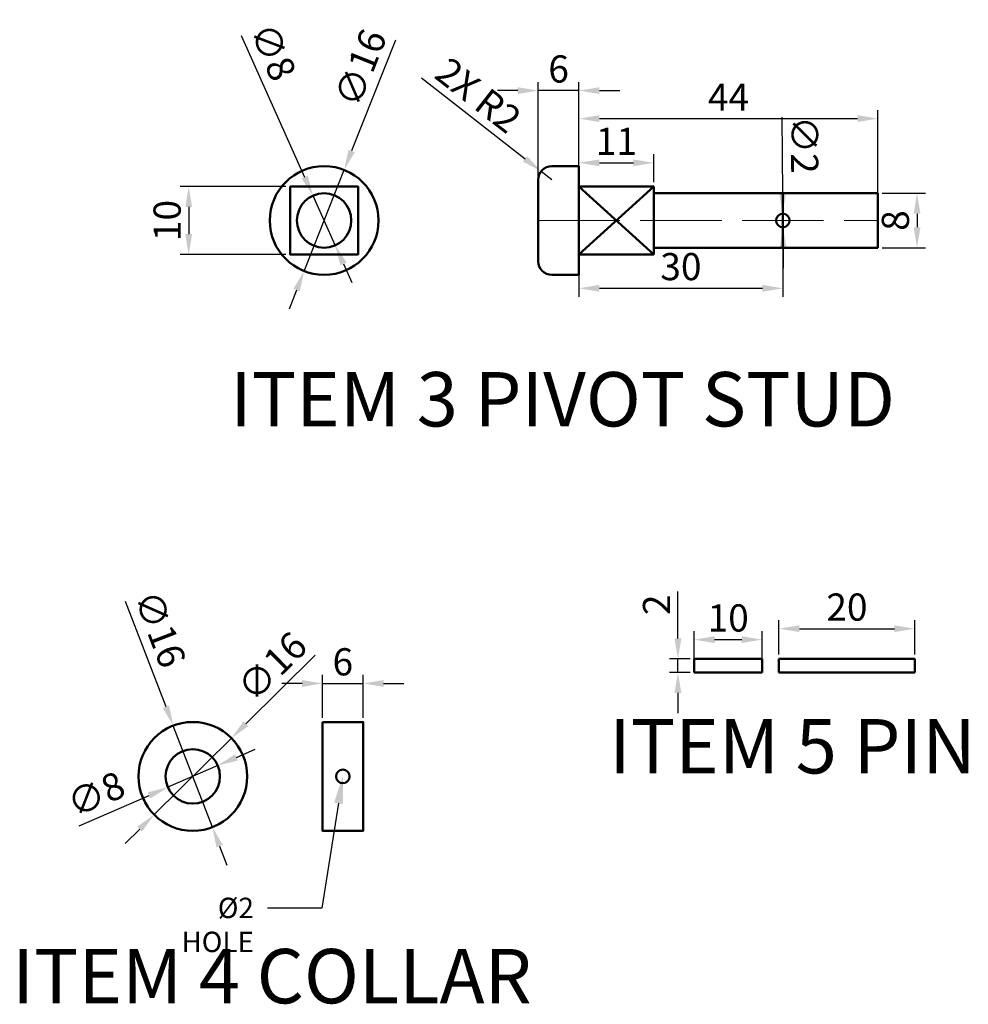
# Model space of a CAD drawing. Units: millimetres. Extents: x 867 to 1199, y -58 to 305.
# Tile 2 of 3: x 1060 to 1199, y -15 to 130. Entities that reach past the tile are written whole.
import ezdxf
from ezdxf import colors
from ezdxf.entities.mleader import LeaderData, LeaderLine
from ezdxf.math import Vec2, Vec3

# ---------------------------------------------------------------- set-up
doc = ezdxf.new("R2010")
doc.units = ezdxf.units.MM
doc.linetypes.add('ACAD_ISO02W100', pattern=[15, 12, -3])
for name, color, linetype, lineweight in [('M-CNTR', 1, 'ACAD_ISO02W100', 18), ('M-DIMS', 2, 'Continuous', 25), ('M-OUTL', 7, 'Continuous', 50), ('M-TEXT', 3, 'Continuous', 25)]:
    doc.layers.add(name, color=color, linetype=linetype, lineweight=lineweight)
doc.styles.get("Standard").update_dxf_attribs({"font": 'arial.ttf'})
doc.dimstyles.new('ISO-25', dxfattribs={"dimtxt": 4, "dimasz": 3, "dimexe": 1.25, "dimexo": 0.625, "dimtad": 1, "dimdec": 1, "dimtxsty": 'Standard', "dimcen": 2.5, "dimadec": 0, "dimazin": 0, "dimtfac": 1, "dimtdec": 1, "dimtmove": 0, "dimatfit": 3, "dimfxl": 1, "dimarcsym": 0})

# ---------------------------------------------------------------- blocks, each defined once
blk = doc.blocks.new('*D35')
at = {"layer": 'Defpoints', "color": 0, "transparency": 16777216}
for p in [(1136.01, 119.83), (1136.01, 100.72), (1142.01, 100.72)]:
    blk.add_point(p, dxfattribs=at)
at = {"layer": 'M-DIMS', "color": 0, "lineweight": -2, "transparency": 16777216}
for p, q in [((1136.01, 101.35), (1136.01, 121.08)), ((1142.01, 101.35), (1142.01, 121.08)), ((1133.01, 119.83), (1130.01, 119.83)), ((1142.01, 119.83), (1136.01, 119.83)), ((1145.01, 119.83), (1148.01, 119.83))]:
    blk.add_line(p, q, dxfattribs=at)
at = {"layer": 'M-DIMS', "color": 0, "transparency": 16777216}
for points in [[(1133.01, 120.33), (1133.01, 119.33), (1136.01, 119.83)], [(1145.01, 120.33), (1145.01, 119.33), (1142.01, 119.83)]]:
    blk.add_solid(points, dxfattribs=at)
at = {"layer": 'M-DIMS', "color": 0, "transparency": 16777216, "insert": (1139.01, 122.5), "char_height": 4, "attachment_point": 5}
blk.add_mtext('6', dxfattribs=at)
blk = doc.blocks.new('*D36')
at = {"layer": 'Defpoints', "color": 0, "transparency": 16777216}
for p in [(1186.01, 115.71), (1142.01, 109.67), (1186.01, 100.72)]:
    blk.add_point(p, dxfattribs=at)
at = {"layer": 'M-DIMS', "color": 0, "lineweight": -2, "transparency": 16777216}
for p, q in [((1142.01, 110.3), (1142.01, 116.96)), ((1186.01, 101.35), (1186.01, 116.96)), ((1145.01, 115.71), (1183.01, 115.71))]:
    blk.add_line(p, q, dxfattribs=at)
at = {"layer": 'M-DIMS', "color": 0, "transparency": 16777216}
for points in [[(1145.01, 116.21), (1145.01, 115.21), (1142.01, 115.71)], [(1183.01, 116.21), (1183.01, 115.21), (1186.01, 115.71)]]:
    blk.add_solid(points, dxfattribs=at)
at = {"layer": 'M-DIMS', "color": 0, "transparency": 16777216, "insert": (1164.01, 118.34), "char_height": 4, "attachment_point": 5}
blk.add_mtext('44', dxfattribs=at)
blk = doc.blocks.new('*D37')
at = {"layer": 'Defpoints', "color": 0, "transparency": 16777216}
for p in [(1153.01, 109.21), (1142.01, 105.72), (1153.01, 105.72)]:
    blk.add_point(p, dxfattribs=at)
at = {"layer": 'M-DIMS', "color": 0, "lineweight": -2, "transparency": 16777216}
for p, q in [((1142.01, 106.35), (1142.01, 110.46)), ((1153.01, 106.35), (1153.01, 110.46)), ((1145.01, 109.21), (1150.01, 109.21))]:
    blk.add_line(p, q, dxfattribs=at)
at = {"layer": 'M-DIMS', "color": 0, "transparency": 16777216}
for points in [[(1145.01, 109.71), (1145.01, 108.71), (1142.01, 109.21)], [(1150.01, 109.71), (1150.01, 108.71), (1153.01, 109.21)]]:
    blk.add_solid(points, dxfattribs=at)
at = {"layer": 'M-DIMS', "color": 0, "transparency": 16777216, "insert": (1147.51, 111.85), "char_height": 4, "attachment_point": 5}
blk.add_mtext('11', dxfattribs=at)
blk = doc.blocks.new('*D38')
at = {"layer": 'Defpoints', "color": 0, "transparency": 16777216}
for p in [(1172.01, 100.72), (1142.01, 94.01), (1172.01, 90.75)]:
    blk.add_point(p, dxfattribs=at)
at = {"layer": 'M-DIMS', "color": 0, "lineweight": -2, "transparency": 16777216}
for p, q in [((1172.01, 100.1), (1172.01, 89.5)), ((1142.01, 93.39), (1142.01, 89.5)), ((1145.01, 90.75), (1169.01, 90.75))]:
    blk.add_line(p, q, dxfattribs=at)
at = {"layer": 'M-DIMS', "color": 0, "transparency": 16777216}
for points in [[(1145.01, 91.25), (1145.01, 90.25), (1142.01, 90.75)], [(1169.01, 91.25), (1169.01, 90.25), (1172.01, 90.75)]]:
    blk.add_solid(points, dxfattribs=at)
at = {"layer": 'M-DIMS', "color": 0, "transparency": 16777216, "insert": (1157.01, 93.42), "char_height": 4, "attachment_point": 5}
blk.add_mtext('30', dxfattribs=at)
blk = doc.blocks.new('*D39')
at = {"layer": 'Defpoints', "color": 0, "transparency": 16777216}
for p in [(1107.45, 108.16), (1101.56, 93.28)]:
    blk.add_point(p, dxfattribs=at)
at = {"layer": 'M-DIMS', "color": 0, "lineweight": -2, "transparency": 16777216}
for p, q in [((1115, 127.24), (1108.55, 110.95)), ((1101.56, 93.28), (1107.45, 108.16)), ((1100.46, 90.49), (1099.36, 87.7))]:
    blk.add_line(p, q, dxfattribs=at)
at = {"layer": 'M-DIMS', "color": 0, "transparency": 16777216}
for points in [[(1108.09, 111.13), (1109.02, 110.77), (1107.45, 108.16)], [(1099.99, 90.68), (1100.92, 90.31), (1101.56, 93.28)]]:
    blk.add_solid(points, dxfattribs=at)
at = {"layer": 'M-DIMS', "color": 0, "transparency": 16777216, "insert": (1110.33, 122.99), "char_height": 4, "attachment_point": 5, "rotation": 68.4119}
blk.add_mtext('∅16', dxfattribs=at)
blk = doc.blocks.new('*D40')
at = {"layer": 'Defpoints', "color": 0, "transparency": 16777216}
for p in [(1102.87, 104.37), (1106.14, 97.07)]:
    blk.add_point(p, dxfattribs=at)
at = {"layer": 'M-DIMS', "color": 0, "lineweight": -2, "transparency": 16777216}
for p, q in [((1092.31, 127.94), (1101.64, 107.11)), ((1106.14, 97.07), (1102.87, 104.37)), ((1107.37, 94.33), (1108.59, 91.6))]:
    blk.add_line(p, q, dxfattribs=at)
at = {"layer": 'M-DIMS', "color": 0, "transparency": 16777216}
for points in [[(1102.1, 107.31), (1101.19, 106.91), (1102.87, 104.37)], [(1107.82, 94.54), (1106.91, 94.13), (1106.14, 97.07)]]:
    blk.add_solid(points, dxfattribs=at)
at = {"layer": 'M-DIMS', "color": 0, "transparency": 16777216, "insert": (1096.53, 125.32), "char_height": 4, "attachment_point": 5, "rotation": 294.1315}
blk.add_mtext('∅8', dxfattribs=at)
blk = doc.blocks.new('*D41')
at = {"layer": 'Defpoints', "color": 0, "transparency": 16777216}
for p in [(1099.51, 105.72), (1084.58, 95.72), (1099.51, 95.72)]:
    blk.add_point(p, dxfattribs=at)
at = {"layer": 'M-DIMS', "color": 0, "lineweight": -2, "transparency": 16777216}
for p, q in [((1098.88, 105.72), (1083.33, 105.72)), ((1084.58, 102.72), (1084.58, 98.72)), ((1098.88, 95.72), (1083.33, 95.72))]:
    blk.add_line(p, q, dxfattribs=at)
at = {"layer": 'M-DIMS', "color": 0, "transparency": 16777216}
for points in [[(1084.08, 102.72), (1085.08, 102.72), (1084.58, 105.72)], [(1084.08, 98.72), (1085.08, 98.72), (1084.58, 95.72)]]:
    blk.add_solid(points, dxfattribs=at)
at = {"layer": 'M-DIMS', "color": 0, "transparency": 16777216, "insert": (1081.92, 100.72), "char_height": 4, "attachment_point": 5, "rotation": 90}
blk.add_mtext('10', dxfattribs=at)
blk = doc.blocks.new('*D42')
at = {"layer": 'Defpoints', "color": 0, "transparency": 16777216}
for p in [(1110.26, 32.61), (1104.26, 26.94), (1110.26, 26.94)]:
    blk.add_point(p, dxfattribs=at)
at = {"layer": 'M-DIMS', "color": 0, "lineweight": -2, "transparency": 16777216}
for p, q in [((1104.26, 27.56), (1104.26, 33.86)), ((1110.26, 27.56), (1110.26, 33.86)), ((1101.26, 32.61), (1098.26, 32.61)), ((1104.26, 32.61), (1110.26, 32.61)), ((1113.26, 32.61), (1116.26, 32.61))]:
    blk.add_line(p, q, dxfattribs=at)
at = {"layer": 'M-DIMS', "color": 0, "transparency": 16777216}
for points in [[(1101.26, 33.11), (1101.26, 32.11), (1104.26, 32.61)], [(1113.26, 33.11), (1113.26, 32.11), (1110.26, 32.61)]]:
    blk.add_solid(points, dxfattribs=at)
at = {"layer": 'M-DIMS', "color": 0, "transparency": 16777216, "insert": (1107.26, 35.28), "char_height": 4, "attachment_point": 5}
blk.add_mtext('6', dxfattribs=at)
blk = doc.blocks.new('*D43')
at = {"layer": 'Defpoints', "color": 0, "transparency": 16777216}
for p in [(1082.31, 26.4), (1088.06, 11.47)]:
    blk.add_point(p, dxfattribs=at)
at = {"layer": 'M-DIMS', "color": 0, "lineweight": -2, "transparency": 16777216}
for p, q in [((1075.25, 44.72), (1081.23, 29.2)), ((1088.06, 11.47), (1082.31, 26.4)), ((1089.13, 8.67), (1090.21, 5.87))]:
    blk.add_line(p, q, dxfattribs=at)
at = {"layer": 'M-DIMS', "color": 0, "transparency": 16777216}
for points in [[(1081.69, 29.38), (1080.76, 29.02), (1082.31, 26.4)], [(1089.6, 8.85), (1088.67, 8.49), (1088.06, 11.47)]]:
    blk.add_solid(points, dxfattribs=at)
at = {"layer": 'M-DIMS', "color": 0, "transparency": 16777216, "insert": (1079.88, 40.44), "char_height": 4, "attachment_point": 5, "rotation": 291.0664}
blk.add_mtext('∅16', dxfattribs=at)
blk = doc.blocks.new('*D44')
at = {"layer": 'Defpoints', "color": 0, "transparency": 16777216}
for p in [(1088.85, 20.53), (1081.51, 17.34)]:
    blk.add_point(p, dxfattribs=at)
at = {"layer": 'M-DIMS', "color": 0, "lineweight": -2, "transparency": 16777216}
for p, q in [((1091.6, 21.73), (1094.35, 22.93)), ((1088.85, 20.53), (1081.51, 17.34)), ((1068.47, 11.65), (1078.76, 16.14))]:
    blk.add_line(p, q, dxfattribs=at)
at = {"layer": 'M-DIMS', "color": 0, "transparency": 16777216}
for points in [[(1091.4, 22.19), (1091.8, 21.27), (1088.85, 20.53)], [(1078.56, 16.6), (1078.96, 15.68), (1081.51, 17.34)]]:
    blk.add_solid(points, dxfattribs=at)
at = {"layer": 'M-DIMS', "color": 0, "transparency": 16777216, "insert": (1071.13, 15.85), "char_height": 4, "attachment_point": 5, "rotation": 23.542}
blk.add_mtext('∅8', dxfattribs=at)
blk = doc.blocks.new('*D45')
at = {"layer": 'Defpoints', "color": 0, "transparency": 16777216}
for p in [(1191.44, 40.67), (1171.44, 36.23), (1191.44, 36.23)]:
    blk.add_point(p, dxfattribs=at)
at = {"layer": 'M-DIMS', "color": 0, "lineweight": -2, "transparency": 16777216}
for p, q in [((1171.44, 36.86), (1171.44, 41.92)), ((1174.44, 40.67), (1188.44, 40.67)), ((1191.44, 36.86), (1191.44, 41.92))]:
    blk.add_line(p, q, dxfattribs=at)
at = {"layer": 'M-DIMS', "color": 0, "transparency": 16777216}
for points in [[(1174.44, 41.17), (1174.44, 40.17), (1171.44, 40.67)], [(1188.44, 41.17), (1188.44, 40.17), (1191.44, 40.67)]]:
    blk.add_solid(points, dxfattribs=at)
at = {"layer": 'M-DIMS', "color": 0, "transparency": 16777216, "insert": (1181.44, 43.33), "char_height": 4, "attachment_point": 5}
blk.add_mtext('20', dxfattribs=at)
blk = doc.blocks.new('*D46')
at = {"layer": 'Defpoints', "color": 0, "transparency": 16777216}
for p in [(1156.57, 36.23), (1158.97, 36.23), (1158.97, 34.23)]:
    blk.add_point(p, dxfattribs=at)
at = {"layer": 'M-DIMS', "color": 0, "lineweight": -2, "transparency": 16777216}
for p, q in [((1156.57, 39.23), (1156.57, 46.13)), ((1158.35, 36.23), (1155.32, 36.23)), ((1156.57, 34.23), (1156.57, 36.23)), ((1158.35, 34.23), (1155.32, 34.23)), ((1156.57, 31.23), (1156.57, 28.23))]:
    blk.add_line(p, q, dxfattribs=at)
at = {"layer": 'M-DIMS', "color": 0, "transparency": 16777216}
for points in [[(1156.07, 39.23), (1157.07, 39.23), (1156.57, 36.23)], [(1156.07, 31.23), (1157.07, 31.23), (1156.57, 34.23)]]:
    blk.add_solid(points, dxfattribs=at)
at = {"layer": 'M-DIMS', "color": 0, "transparency": 16777216, "insert": (1153.94, 44.18), "char_height": 4, "attachment_point": 5, "rotation": 90}
blk.add_mtext('2', dxfattribs=at)
blk = doc.blocks.new('*D60')
at = {"layer": 'Defpoints', "color": 0, "transparency": 16777216}
for p in [(1186.01, 104.72), (1186.01, 96.72), (1191.76, 96.72)]:
    blk.add_point(p, dxfattribs=at)
at = {"layer": 'M-DIMS', "color": 0, "lineweight": -2, "transparency": 16777216}
for p, q in [((1186.63, 104.72), (1193.01, 104.72)), ((1191.76, 101.72), (1191.76, 99.72)), ((1186.63, 96.72), (1193.01, 96.72))]:
    blk.add_line(p, q, dxfattribs=at)
at = {"layer": 'M-DIMS', "color": 0, "transparency": 16777216}
for points in [[(1191.26, 101.72), (1192.26, 101.72), (1191.76, 104.72)], [(1191.26, 99.72), (1192.26, 99.72), (1191.76, 96.72)]]:
    blk.add_solid(points, dxfattribs=at)
at = {"layer": 'M-DIMS', "color": 0, "transparency": 16777216, "insert": (1189.09, 100.72), "char_height": 4, "attachment_point": 5, "rotation": 90}
blk.add_mtext('8', dxfattribs=at)
blk = doc.blocks.new('*D61')
at = {"layer": 'Defpoints', "color": 0, "transparency": 16777216}
for p in [(1168.97, 39.06), (1158.97, 34.23), (1168.97, 34.23)]:
    blk.add_point(p, dxfattribs=at)
at = {"layer": 'M-DIMS', "color": 0, "lineweight": -2, "transparency": 16777216}
for p, q in [((1158.97, 34.86), (1158.97, 40.31)), ((1168.97, 34.86), (1168.97, 40.31)), ((1161.97, 39.06), (1165.97, 39.06))]:
    blk.add_line(p, q, dxfattribs=at)
at = {"layer": 'M-DIMS', "color": 0, "transparency": 16777216}
for points in [[(1161.97, 39.56), (1161.97, 38.56), (1158.97, 39.06)], [(1165.97, 39.56), (1165.97, 38.56), (1168.97, 39.06)]]:
    blk.add_solid(points, dxfattribs=at)
at = {"layer": 'M-DIMS', "color": 0, "transparency": 16777216, "insert": (1163.97, 41.73), "char_height": 4, "attachment_point": 5}
blk.add_mtext('10', dxfattribs=at)
blk = doc.blocks.new('*D67')
at = {"layer": 'Defpoints', "color": 0, "transparency": 16777216}
for p in [(1172, 101.72), (1172.02, 99.72)]:
    blk.add_point(p, dxfattribs=at)
at = {"layer": 'M-DIMS', "color": 0, "lineweight": -2, "transparency": 16777216}
for p, q in [((1171.86, 115.9), (1171.97, 104.72)), ((1172.02, 99.72), (1172, 101.72)), ((1172.05, 96.72), (1172.08, 93.72))]:
    blk.add_line(p, q, dxfattribs=at)
at = {"layer": 'M-DIMS', "color": 0, "transparency": 16777216}
for points in [[(1172.47, 104.73), (1171.47, 104.72), (1172, 101.72)], [(1172.55, 96.73), (1171.55, 96.72), (1172.02, 99.72)]]:
    blk.add_solid(points, dxfattribs=at)
at = {"layer": 'M-DIMS', "color": 0, "transparency": 16777216, "insert": (1174.68, 111.84), "char_height": 4, "attachment_point": 5, "rotation": 270.5848}
blk.add_mtext('∅2', dxfattribs=at)
blk = doc.blocks.new('*D68')
at = {"layer": 'Defpoints', "color": 0, "transparency": 16777216}
for p in [(1136.43, 107.95), (1138.01, 106.72)]:
    blk.add_point(p, dxfattribs=at)
at = {"layer": 'M-DIMS', "color": 0, "lineweight": -2, "transparency": 16777216}
for p, q in [((1118.84, 121.69), (1134.07, 109.8)), ((1138.01, 106.72), (1136.43, 107.95))]:
    blk.add_line(p, q, dxfattribs=at)
at = {"layer": 'M-DIMS', "color": 0, "transparency": 16777216}
blk.add_solid([(1134.38, 110.19), (1133.76, 109.4), (1136.43, 107.95)], dxfattribs=at)
at = {"layer": 'M-DIMS', "color": 0, "transparency": 16777216, "insert": (1126.89, 118.74), "char_height": 4, "attachment_point": 5, "rotation": 322.0267}
blk.add_mtext('2X R2', dxfattribs=at)
blk = doc.blocks.new('*D69')
at = {"layer": 'Defpoints', "color": 0, "transparency": 16777216}
for p in [(1090.87, 24.57), (1079.5, 13.31)]:
    blk.add_point(p, dxfattribs=at)
at = {"layer": 'M-DIMS', "color": 0, "lineweight": -2, "transparency": 16777216}
for p, q in [((1103.18, 36.76), (1093, 26.68)), ((1079.5, 13.31), (1090.87, 24.57)), ((1077.37, 11.2), (1075.23, 9.08))]:
    blk.add_line(p, q, dxfattribs=at)
at = {"layer": 'M-DIMS', "color": 0, "transparency": 16777216}
for points in [[(1092.64, 27.03), (1093.35, 26.32), (1090.87, 24.57)], [(1077.01, 11.55), (1077.72, 10.84), (1079.5, 13.31)]]:
    blk.add_solid(points, dxfattribs=at)
at = {"layer": 'M-DIMS', "color": 0, "transparency": 16777216, "insert": (1097.2, 34.75), "char_height": 4, "attachment_point": 5, "rotation": 44.7223}
blk.add_mtext('∅16', dxfattribs=at)

msp = doc.modelspace()

# ---------------------------------------------------------------- linework, layer by layer
at = {"layer": 'M-CNTR'}
msp.add_line((1136.01, 100.721), (1186.01, 100.721), dxfattribs=at)
at = {"layer": 'M-OUTL'}
for p, q in [((1142.01, 108.721), (1138.01, 108.721)), ((1142.01, 92.721), (1142.01, 108.721)), ((1136.01, 106.721), (1136.01, 94.721)), ((1142.01, 105.721), (1153.01, 105.721)), ((1142.01, 105.721), (1153.01, 95.721)), ((1153.01, 105.721), (1142.01, 95.721)), ((1153.01, 95.721), (1153.01, 105.721)), ((1153.01, 104.721), (1186.01, 104.721)), ((1172.01, 96.721), (1172.01, 104.721)), ((1186.01, 96.721), (1186.01, 104.721)), ((1142.01, 95.721), (1153.01, 95.721)), ((1153.01, 96.721), (1186.01, 96.721)), ((1138.01, 92.721), (1142.01, 92.721)), ((1158.97, 34.232), (1158.97, 36.232)), ((1158.97, 36.232), (1168.97, 36.232)), ((1168.97, 36.232), (1168.97, 34.232)), ((1171.439, 36.232), (1191.439, 36.232)), ((1171.439, 34.232), (1171.439, 36.232)), ((1191.439, 36.232), (1191.439, 34.232)), ((1168.97, 34.232), (1158.97, 34.232)), ((1191.439, 34.232), (1171.439, 34.232))]:
    msp.add_line(p, q, dxfattribs=at)
for points in [[(1099.506, 105.721), (1109.506, 105.721), (1109.506, 95.721), (1099.506, 95.721)], [(1104.258, 26.936), (1110.258, 26.936), (1110.258, 10.936), (1104.258, 10.936)]]:
    msp.add_lwpolyline(points, close=True, dxfattribs=at)
for centre, radius in [((1104.506, 100.721), 8), ((1104.506, 100.721), 4), ((1172.01, 100.721), 1), ((1085.181, 18.936), 8), ((1085.181, 18.936), 4), ((1107.258, 18.936), 1)]:
    msp.add_circle(centre, radius, dxfattribs=at)
for centre, start, end in [((1138.01, 106.721), 90, 180), ((1138.01, 94.721), 180, 270)]:
    msp.add_arc(centre, 2, start, end, dxfattribs=at)

# ---------------------------------------------------------------- texts
at = {"layer": 'M-TEXT', "char_height": 8, "attachment_point": 1}
for s, insert in [('ITEM 3 PIVOT STUD', (1090.664, 78.426)), ('     ITEM 5 PIN', (1134.212, 27.373)), ('ITEM 4 COLLAR', (1058.603, -6.449))]:
    msp.add_mtext_dynamic_manual_height_columns(s, width=111.81004, gutter_width=12.5, heights=[0], dxfattribs=dict(at, insert=insert))

# ---------------------------------------------------------------- dimensions: what is measured, and where the dimension line sits
at = {"layer": 'M-DIMS'}
for p1, p2, picture, middle in [((1106.142, 97.071), (1102.871, 104.372), '*D40', (1093.996, 124.183)), ((1101.563, 93.283), (1107.45, 108.16), '*D39', (1112.914, 121.97)), ((1088.057, 11.471), (1082.305, 26.401), '*D43', (1077.284, 39.439))]:
    dim = msp.add_diameter_dim_2p(p1=p1, p2=p2, dimstyle='ISO-25', override={"dimclrd": 0, "dimclre": 0, "dimclrt": 0}, dxfattribs=at)
    dim.commit()
    dim.dimension.update_dxf_attribs({"geometry": picture, "text_midpoint": middle, "dimtype": 163})
dim = msp.add_radius_dim(center=(1138.01, 106.721), mpoint=(1136.433, 107.952), text='2X <>', dimstyle='ISO-25', override={"dimdec": 0, "dimlfac": 1, "dimrnd": 0, "dimzin": 0, "dimdsep": 46, "dimlunit": 2}, dxfattribs=at)
dim.commit()
dim.dimension.update_dxf_attribs({"geometry": '*D68', "text_midpoint": (1126.891, 118.742)})
for base, p1, p2, override, picture, middle in [((1136.01, 119.832), (1142.01, 100.721), (1136.01, 100.721), {"dimclrd": 0, "dimclre": 0, "dimclrt": 0}, '*D35', (1139.01, 122.499)), ((1186.01, 115.712), (1142.01, 109.67), (1186.01, 100.721), {"dimclrd": 0, "dimclre": 0, "dimclrt": 0}, '*D36', (1164.01, 118.337)), ((1153.01, 109.212), (1142.01, 105.721), (1153.01, 105.721), {"dimclrd": 0, "dimclre": 0, "dimclrt": 0}, '*D37', (1147.51, 111.845)), ((1172.01, 90.754), (1142.01, 94.015), (1172.01, 100.721), {"dimclrd": 0, "dimclre": 0, "dimclrt": 0}, '*D38', (1157.01, 93.423)), ((1191.439, 40.665), (1171.439, 36.232), (1191.439, 36.232), {"dimclrd": 0, "dimclre": 0, "dimclrt": 0}, '*D45', (1181.439, 43.333)), ((1168.97, 39.062), (1158.97, 34.232), (1168.97, 34.232), {"dimdec": 0, "dimlfac": 1, "dimrnd": 0, "dimzin": 0, "dimdsep": 46, "dimlunit": 2}, '*D61', (1163.97, 41.729)), ((1110.258, 32.61), (1104.258, 26.936), (1110.258, 26.936), {"dimclrd": 0, "dimclre": 0, "dimclrt": 0}, '*D42', (1107.258, 35.278))]:
    dim = msp.add_linear_dim(base=base, p1=p1, p2=p2, dimstyle='ISO-25', override=override, dxfattribs=at)
    dim.commit()
    dim.dimension.update_dxf_attribs({"geometry": picture, "text_midpoint": middle})
for p1, p2, override, picture, middle in [((1172.02, 99.721), (1172, 101.721), {"dimdec": 0, "dimlfac": 1, "dimrnd": 0, "dimzin": 0, "dimdsep": 46, "dimlunit": 2}, '*D67', (1171.897, 111.812)), ((1079.497, 13.307), (1090.865, 24.566), {"dimdec": 0, "dimlfac": 1, "dimrnd": 0, "dimzin": 0, "dimdsep": 46, "dimlunit": 2}, '*D69', (1099.153, 32.774)), ((1088.848, 20.534), (1081.514, 17.338), {"dimclrd": 0, "dimclre": 0, "dimclrt": 0}, '*D44', (1071.13, 15.846))]:
    dim = msp.add_diameter_dim_2p(p1=p1, p2=p2, dimstyle='ISO-25', override=override, dxfattribs=at)
    dim.commit()
    dim.dimension.update_dxf_attribs({"geometry": picture, "text_midpoint": middle})
for base, p1, p2, override, picture, middle in [((1084.583, 95.721), (1099.506, 105.721), (1099.506, 95.721), {"dimclrd": 0, "dimclre": 0, "dimclrt": 0}, '*D41', (1081.915, 100.721)), ((1191.76, 96.721), (1186.01, 104.721), (1186.01, 96.721), {"dimdec": 0, "dimlfac": 1, "dimrnd": 0, "dimzin": 0, "dimdsep": 46, "dimlunit": 2}, '*D60', (1189.093, 100.721)), ((1156.574, 36.232), (1158.97, 34.232), (1158.97, 36.232), {"dimclrd": 0, "dimclre": 0, "dimclrt": 0}, '*D46', (1153.941, 44.181))]:
    dim = msp.add_linear_dim(base=base, p1=p1, p2=p2, angle=90, dimstyle='ISO-25', override=override, dxfattribs=at)
    dim.commit()
    dim.dimension.update_dxf_attribs({"geometry": picture, "text_midpoint": middle})

# ---------------------------------------------------------------- leaders
at = {"layer": 'M-TEXT'}
ml = msp.add_multileader_mtext('Standard', dxfattribs=at)
ml.set_content('\\pxi-3,l4,t4;%%C2 HOLE', color=256)
ml.set_leader_properties()
ml.build(insert=Vec2(0, 0))
ctx = ml.context
ctx.base_point, ctx.char_height, ctx.plane_origin = Vec3(1074.392, -0.469), 3, Vec3(1107.258, 18.936)
ctx.text_align_type = 2
notes = []
notes.append((ctx, [(0, (1, 1, 0), (1104.165, -0.469), (-1, 0), 8, [(0, [(1107.258, 18.936)], 0, [])])]))
ctx.mtext.insert, ctx.mtext.alignment, ctx.mtext.flow_direction = Vec3(1094.165, 1.091), 3, 5
for ctx, leaders in notes:
    for number, flags, end, landing, length, lines in leaders:
        leader = LeaderData()
        leader.index, (leader.has_last_leader_line, leader.has_dogleg_vector, leader.attachment_direction) = number, flags
        leader.last_leader_point, leader.dogleg_vector, leader.dogleg_length = Vec3(end), Vec3(landing), length
        for number, points, colour, breaks in lines:
            line = LeaderLine()
            line.index, line.vertices, line.color, line.breaks = number, Vec3.list(points), colors.encode_raw_color(colour), breaks
            leader.lines.append(line)
        ctx.leaders.append(leader)

doc.saveas('drawing.dxf')
